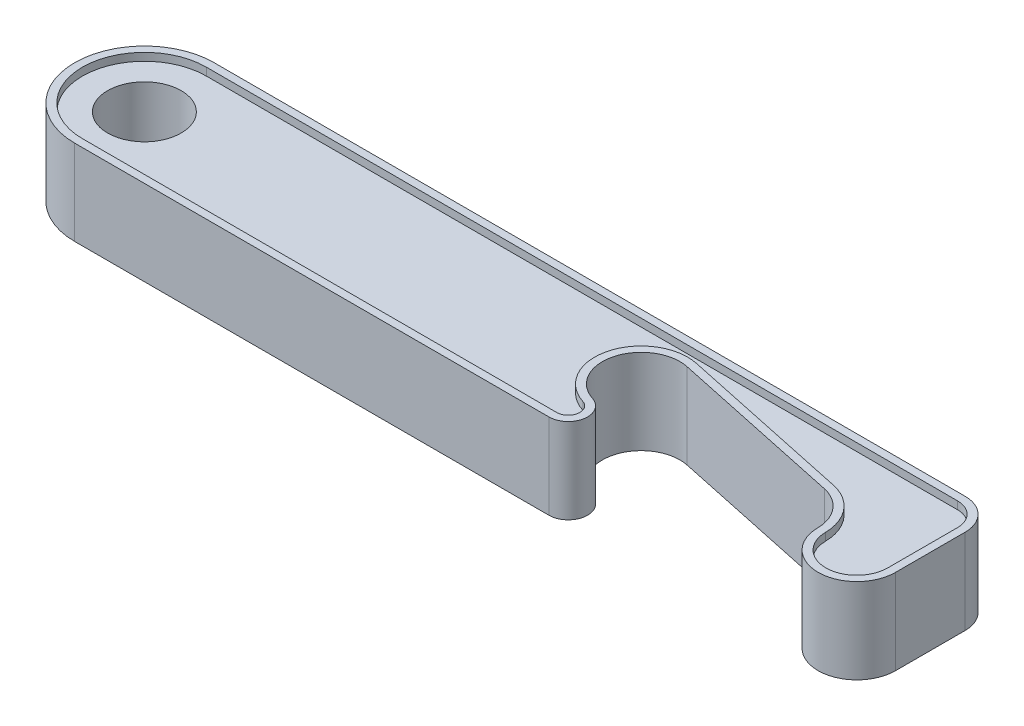
ISO-10303-21;
HEADER;
FILE_DESCRIPTION(('STEP AP214'),'2;1');
FILE_NAME('part.step','',(''),(''),'','','');
FILE_SCHEMA(('AUTOMOTIVE_DESIGN { 1 0 10303 214 1 1 1 1 }'));
ENDSEC;
DATA;
#1=APPLICATION_CONTEXT('core data for automotive mechanical design processes');
#2=APPLICATION_PROTOCOL_DEFINITION('international standard','automotive_design',2000,#1);
#3=PRODUCT_CONTEXT('',#1,'mechanical');
#4=PRODUCT('Part','Part','',(#3));
#5=PRODUCT_RELATED_PRODUCT_CATEGORY('part','',(#4));
#6=PRODUCT_DEFINITION_FORMATION('','',#4);
#7=PRODUCT_DEFINITION_CONTEXT('part definition',#1,'design');
#8=PRODUCT_DEFINITION('design','',#6,#7);
#9=PRODUCT_DEFINITION_SHAPE('','',#8);
#10=(LENGTH_UNIT() NAMED_UNIT(*) SI_UNIT(.MILLI.,.METRE.));
#11=(NAMED_UNIT(*) PLANE_ANGLE_UNIT() SI_UNIT($,.RADIAN.));
#12=(NAMED_UNIT(*) SI_UNIT($,.STERADIAN.) SOLID_ANGLE_UNIT());
#13=UNCERTAINTY_MEASURE_WITH_UNIT(LENGTH_MEASURE(1.E-05),#10,'distance_accuracy_value','');
#14=(GEOMETRIC_REPRESENTATION_CONTEXT(3) GLOBAL_UNCERTAINTY_ASSIGNED_CONTEXT((#13)) GLOBAL_UNIT_ASSIGNED_CONTEXT((#10,
#11,#12)) REPRESENTATION_CONTEXT('',''));
#15=CARTESIAN_POINT('',(0.,0.,0.));
#16=DIRECTION('',(0.,0.,1.));
#17=DIRECTION('',(1.,0.,0.));
#18=AXIS2_PLACEMENT_3D('',#15,#16,#17);
#19=CARTESIAN_POINT('',(0.,4.5,0.));
#20=DIRECTION('',(0.,-1.,0.));
#21=DIRECTION('',(0.,0.,-1.));
#22=AXIS2_PLACEMENT_3D('',#19,#20,#21);
#23=CYLINDRICAL_SURFACE('',#22,4.75);
#24=CARTESIAN_POINT('',(0.,4.5,0.));
#25=DIRECTION('',(0.,1.,0.));
#26=DIRECTION('',(0.,0.,1.));
#27=AXIS2_PLACEMENT_3D('',#24,#25,#26);
#28=CIRCLE('',#27,4.75);
#29=CARTESIAN_POINT('',(0.,4.5,4.75));
#30=VERTEX_POINT('',#29);
#31=EDGE_CURVE('E97',#30,#30,#28,.T.);
#32=ORIENTED_EDGE('',*,*,#31,.T.);
#33=EDGE_LOOP('',(#32));
#34=FACE_BOUND('',#33,.T.);
#35=CARTESIAN_POINT('',(0.,-4.5,0.));
#36=DIRECTION('',(0.,1.,0.));
#37=DIRECTION('',(0.,0.,1.));
#38=AXIS2_PLACEMENT_3D('',#35,#36,#37);
#39=CIRCLE('',#38,4.75);
#40=CARTESIAN_POINT('',(0.,-4.5,4.75));
#41=VERTEX_POINT('',#40);
#42=EDGE_CURVE('E159',#41,#41,#39,.T.);
#43=ORIENTED_EDGE('',*,*,#42,.F.);
#44=EDGE_LOOP('',(#43));
#45=FACE_BOUND('',#44,.T.);
#46=ADVANCED_FACE('F41',(#34,#45),#23,.F.);
#47=CARTESIAN_POINT('',(0.,4.5,0.));
#48=DIRECTION('',(0.,1.,0.));
#49=DIRECTION('',(0.,0.,1.));
#50=AXIS2_PLACEMENT_3D('',#47,#48,#49);
#51=PLANE('',#50);
#52=ORIENTED_EDGE('',*,*,#31,.F.);
#53=EDGE_LOOP('',(#52));
#54=FACE_BOUND('',#53,.T.);
#55=CARTESIAN_POINT('',(86.0008864599619,4.5,4.13314808832979));
#56=DIRECTION('',(0.,1.,0.));
#57=DIRECTION('',(0.,0.,1.));
#58=AXIS2_PLACEMENT_3D('',#55,#56,#57);
#59=CIRCLE('',#58,6.);
#60=CARTESIAN_POINT('',(92.0003545839848,4.5,4.05325923533293));
#61=VERTEX_POINT('',#60);
#62=CARTESIAN_POINT('',(87.2483566048684,4.5,-1.73573751607304));
#63=VERTEX_POINT('',#62);
#64=EDGE_CURVE('E133',#61,#63,#59,.T.);
#65=ORIENTED_EDGE('',*,*,#64,.F.);
#66=CARTESIAN_POINT('',(96.,4.5,4.));
#67=DIRECTION('',(0.,1.,0.));
#68=DIRECTION('',(0.,0.,1.));
#69=AXIS2_PLACEMENT_3D('',#66,#67,#68);
#70=CIRCLE('',#69,4.);
#71=CARTESIAN_POINT('',(100.,4.5,3.99999999999996));
#72=VERTEX_POINT('',#71);
#73=EDGE_CURVE('E140',#61,#72,#70,.T.);
#74=ORIENTED_EDGE('',*,*,#73,.T.);
#75=DIRECTION('',(0.,0.,-1.));
#76=VECTOR('',#75,1.);
#77=CARTESIAN_POINT('',(100.,4.5,0.));
#78=LINE('',#77,#76);
#79=CARTESIAN_POINT('',(100.,4.5,-4.99999999999997));
#80=VERTEX_POINT('',#79);
#81=EDGE_CURVE('E136',#72,#80,#78,.T.);
#82=ORIENTED_EDGE('',*,*,#81,.T.);
#83=CARTESIAN_POINT('',(97.,4.5,-5.));
#84=DIRECTION('',(0.,1.,0.));
#85=DIRECTION('',(0.,0.,1.));
#86=AXIS2_PLACEMENT_3D('',#83,#84,#85);
#87=CIRCLE('',#86,3.);
#88=CARTESIAN_POINT('',(97.,4.5,-8.));
#89=VERTEX_POINT('',#88);
#90=EDGE_CURVE('E141',#80,#89,#87,.T.);
#91=ORIENTED_EDGE('',*,*,#90,.T.);
#92=DIRECTION('',(1.,0.,0.));
#93=VECTOR('',#92,1.);
#94=CARTESIAN_POINT('',(0.,4.5,-8.));
#95=LINE('',#94,#93);
#96=CARTESIAN_POINT('',(0.,4.5,-8.));
#97=VERTEX_POINT('',#96);
#98=EDGE_CURVE('E148',#97,#89,#95,.T.);
#99=ORIENTED_EDGE('',*,*,#98,.F.);
#100=CARTESIAN_POINT('',(0.,4.5,0.));
#101=DIRECTION('',(0.,1.,0.));
#102=DIRECTION('',(0.,0.,1.));
#103=AXIS2_PLACEMENT_3D('',#100,#101,#102);
#104=CIRCLE('',#103,8.);
#105=CARTESIAN_POINT('',(0.,4.5,8.));
#106=VERTEX_POINT('',#105);
#107=EDGE_CURVE('E149',#97,#106,#104,.T.);
#108=ORIENTED_EDGE('',*,*,#107,.T.);
#109=DIRECTION('',(1.,0.,0.));
#110=VECTOR('',#109,1.);
#111=CARTESIAN_POINT('',(0.,4.5,8.));
#112=LINE('',#111,#110);
#113=CARTESIAN_POINT('',(61.234514126342,4.5,8.));
#114=VERTEX_POINT('',#113);
#115=EDGE_CURVE('E155',#106,#114,#112,.T.);
#116=ORIENTED_EDGE('',*,*,#115,.T.);
#117=CARTESIAN_POINT('',(61.234514126342,4.5,6.5));
#118=DIRECTION('',(0.,1.,0.));
#119=DIRECTION('',(0.,0.,1.));
#120=AXIS2_PLACEMENT_3D('',#117,#118,#119);
#121=CIRCLE('',#120,1.5);
#122=CARTESIAN_POINT('',(61.687788593066,4.5,5.07012509015086));
#123=VERTEX_POINT('',#122);
#124=EDGE_CURVE('E154',#114,#123,#121,.T.);
#125=ORIENTED_EDGE('',*,*,#124,.T.);
#126=CARTESIAN_POINT('',(63.5008864599619,4.5,-0.649374549245707));
#127=DIRECTION('',(0.,1.,0.));
#128=DIRECTION('',(0.,0.,1.));
#129=AXIS2_PLACEMENT_3D('',#126,#127,#128);
#130=CIRCLE('',#129,6.);
#131=CARTESIAN_POINT('',(64.7483566048684,4.5,-6.51826015364854));
#132=VERTEX_POINT('',#131);
#133=EDGE_CURVE('E49',#132,#123,#130,.T.);
#134=ORIENTED_EDGE('',*,*,#133,.F.);
#135=DIRECTION('',(0.978147600733806,0.,0.20791169081776));
#136=VECTOR('',#135,1.);
#137=CARTESIAN_POINT('',(4.12450239612868,4.5,-19.404258159443));
#138=LINE('',#137,#136);
#139=EDGE_CURVE('E11',#132,#63,#138,.T.);
#140=ORIENTED_EDGE('',*,*,#139,.T.);
#141=EDGE_LOOP('',(#65,#74,#82,#91,#99,#108,#116,#125,#134,#140));
#142=FACE_BOUND('',#141,.T.);
#143=ADVANCED_FACE('F232',(#54,#142),#51,.T.);
#144=CARTESIAN_POINT('',(0.,-4.5,0.));
#145=DIRECTION('',(0.,1.,0.));
#146=DIRECTION('',(0.,0.,1.));
#147=AXIS2_PLACEMENT_3D('',#144,#145,#146);
#148=PLANE('',#147);
#149=ORIENTED_EDGE('',*,*,#42,.T.);
#150=EDGE_LOOP('',(#149));
#151=FACE_BOUND('',#150,.T.);
#152=CARTESIAN_POINT('',(86.0008864599619,-4.5,4.13314808832979));
#153=DIRECTION('',(0.,1.,0.));
#154=DIRECTION('',(0.,0.,1.));
#155=AXIS2_PLACEMENT_3D('',#152,#153,#154);
#156=CIRCLE('',#155,6.);
#157=CARTESIAN_POINT('',(92.0003545839848,-4.5,4.05325923533293));
#158=VERTEX_POINT('',#157);
#159=CARTESIAN_POINT('',(87.2483566048684,-4.5,-1.73573751607304));
#160=VERTEX_POINT('',#159);
#161=EDGE_CURVE('E94',#158,#160,#156,.T.);
#162=ORIENTED_EDGE('',*,*,#161,.T.);
#163=DIRECTION('',(0.978147600733806,0.,0.20791169081776));
#164=VECTOR('',#163,1.);
#165=CARTESIAN_POINT('',(4.12450239612868,-4.5,-19.404258159443));
#166=LINE('',#165,#164);
#167=CARTESIAN_POINT('',(64.7483566048684,-4.5,-6.51826015364854));
#168=VERTEX_POINT('',#167);
#169=EDGE_CURVE('E42',#168,#160,#166,.T.);
#170=ORIENTED_EDGE('',*,*,#169,.F.);
#171=CARTESIAN_POINT('',(63.5008864599619,-4.5,-0.649374549245707));
#172=DIRECTION('',(0.,1.,0.));
#173=DIRECTION('',(0.,0.,1.));
#174=AXIS2_PLACEMENT_3D('',#171,#172,#173);
#175=CIRCLE('',#174,6.);
#176=CARTESIAN_POINT('',(61.687788593066,-4.5,5.07012509015086));
#177=VERTEX_POINT('',#176);
#178=EDGE_CURVE('E93',#168,#177,#175,.T.);
#179=ORIENTED_EDGE('',*,*,#178,.T.);
#180=CARTESIAN_POINT('',(61.234514126342,-4.5,6.5));
#181=DIRECTION('',(0.,1.,0.));
#182=DIRECTION('',(0.,0.,1.));
#183=AXIS2_PLACEMENT_3D('',#180,#181,#182);
#184=CIRCLE('',#183,1.5);
#185=CARTESIAN_POINT('',(61.234514126342,-4.5,8.));
#186=VERTEX_POINT('',#185);
#187=EDGE_CURVE('E109',#186,#177,#184,.T.);
#188=ORIENTED_EDGE('',*,*,#187,.F.);
#189=DIRECTION('',(1.,0.,0.));
#190=VECTOR('',#189,1.);
#191=CARTESIAN_POINT('',(0.,-4.5,8.));
#192=LINE('',#191,#190);
#193=CARTESIAN_POINT('',(0.,-4.5,8.));
#194=VERTEX_POINT('',#193);
#195=EDGE_CURVE('E179',#194,#186,#192,.T.);
#196=ORIENTED_EDGE('',*,*,#195,.F.);
#197=CARTESIAN_POINT('',(0.,-4.5,0.));
#198=DIRECTION('',(0.,1.,0.));
#199=DIRECTION('',(0.,0.,1.));
#200=AXIS2_PLACEMENT_3D('',#197,#198,#199);
#201=CIRCLE('',#200,8.);
#202=CARTESIAN_POINT('',(0.,-4.5,-8.));
#203=VERTEX_POINT('',#202);
#204=EDGE_CURVE('E177',#203,#194,#201,.T.);
#205=ORIENTED_EDGE('',*,*,#204,.F.);
#206=DIRECTION('',(1.,0.,0.));
#207=VECTOR('',#206,1.);
#208=CARTESIAN_POINT('',(0.,-4.5,-8.));
#209=LINE('',#208,#207);
#210=CARTESIAN_POINT('',(97.,-4.5,-8.));
#211=VERTEX_POINT('',#210);
#212=EDGE_CURVE('E173',#203,#211,#209,.T.);
#213=ORIENTED_EDGE('',*,*,#212,.T.);
#214=CARTESIAN_POINT('',(97.,-4.5,-5.));
#215=DIRECTION('',(0.,1.,0.));
#216=DIRECTION('',(0.,0.,1.));
#217=AXIS2_PLACEMENT_3D('',#214,#215,#216);
#218=CIRCLE('',#217,3.);
#219=CARTESIAN_POINT('',(100.,-4.5,-4.99999999999997));
#220=VERTEX_POINT('',#219);
#221=EDGE_CURVE('E171',#220,#211,#218,.T.);
#222=ORIENTED_EDGE('',*,*,#221,.F.);
#223=DIRECTION('',(0.,0.,-1.));
#224=VECTOR('',#223,1.);
#225=CARTESIAN_POINT('',(100.,-4.5,0.));
#226=LINE('',#225,#224);
#227=CARTESIAN_POINT('',(100.,-4.5,3.99999999999996));
#228=VERTEX_POINT('',#227);
#229=EDGE_CURVE('E169',#228,#220,#226,.T.);
#230=ORIENTED_EDGE('',*,*,#229,.F.);
#231=CARTESIAN_POINT('',(96.,-4.5,4.));
#232=DIRECTION('',(0.,1.,0.));
#233=DIRECTION('',(0.,0.,1.));
#234=AXIS2_PLACEMENT_3D('',#231,#232,#233);
#235=CIRCLE('',#234,4.);
#236=EDGE_CURVE('E164',#158,#228,#235,.T.);
#237=ORIENTED_EDGE('',*,*,#236,.F.);
#238=EDGE_LOOP('',(#162,#170,#179,#188,#196,#205,#213,#222,#230,#237));
#239=FACE_BOUND('',#238,.T.);
#240=ADVANCED_FACE('F89',(#151,#239),#148,.F.);
#241=CARTESIAN_POINT('',(96.,5.5,4.));
#242=DIRECTION('',(0.,-1.,0.));
#243=DIRECTION('',(0.,0.,-1.));
#244=AXIS2_PLACEMENT_3D('',#241,#242,#243);
#245=CYLINDRICAL_SURFACE('',#244,4.);
#246=ORIENTED_EDGE('',*,*,#236,.T.);
#247=DIRECTION('',(0.,-1.,0.));
#248=VECTOR('',#247,1.);
#249=CARTESIAN_POINT('',(100.,5.5,3.99999999999996));
#250=LINE('',#249,#248);
#251=CARTESIAN_POINT('',(100.,-5.5,3.99999999999996));
#252=VERTEX_POINT('',#251);
#253=EDGE_CURVE('E303',#228,#252,#250,.T.);
#254=ORIENTED_EDGE('',*,*,#253,.T.);
#255=CARTESIAN_POINT('',(96.,-5.5,4.));
#256=DIRECTION('',(0.,1.,0.));
#257=DIRECTION('',(0.,0.,1.));
#258=AXIS2_PLACEMENT_3D('',#255,#256,#257);
#259=CIRCLE('',#258,4.);
#260=CARTESIAN_POINT('',(92.0003545839848,-5.5,4.05325923533293));
#261=VERTEX_POINT('',#260);
#262=EDGE_CURVE('E304',#261,#252,#259,.T.);
#263=ORIENTED_EDGE('',*,*,#262,.F.);
#264=DIRECTION('',(0.,-1.,0.));
#265=VECTOR('',#264,1.);
#266=CARTESIAN_POINT('',(92.0003545839848,5.5,4.05325923533293));
#267=LINE('',#266,#265);
#268=EDGE_CURVE('E130',#158,#261,#267,.T.);
#269=ORIENTED_EDGE('',*,*,#268,.F.);
#270=EDGE_LOOP('',(#246,#254,#263,#269));
#271=FACE_BOUND('',#270,.T.);
#272=ADVANCED_FACE('F545',(#271),#245,.F.);
#273=CARTESIAN_POINT('',(86.0008864599619,5.5,4.13314808832979));
#274=DIRECTION('',(0.,-1.,0.));
#275=DIRECTION('',(0.,0.,-1.));
#276=AXIS2_PLACEMENT_3D('',#273,#274,#275);
#277=CYLINDRICAL_SURFACE('',#276,6.);
#278=DIRECTION('',(0.,-1.,0.));
#279=VECTOR('',#278,1.);
#280=CARTESIAN_POINT('',(87.2483566048684,5.5,-1.73573751607304));
#281=LINE('',#280,#279);
#282=CARTESIAN_POINT('',(87.2483566048684,-5.5,-1.73573751607304));
#283=VERTEX_POINT('',#282);
#284=EDGE_CURVE('E118',#160,#283,#281,.T.);
#285=ORIENTED_EDGE('',*,*,#284,.F.);
#286=ORIENTED_EDGE('',*,*,#161,.F.);
#287=ORIENTED_EDGE('',*,*,#268,.T.);
#288=CARTESIAN_POINT('',(86.0008864599619,-5.5,4.13314808832979));
#289=DIRECTION('',(0.,1.,0.));
#290=DIRECTION('',(0.,0.,1.));
#291=AXIS2_PLACEMENT_3D('',#288,#289,#290);
#292=CIRCLE('',#291,6.);
#293=EDGE_CURVE('E307',#261,#283,#292,.T.);
#294=ORIENTED_EDGE('',*,*,#293,.T.);
#295=EDGE_LOOP('',(#285,#286,#287,#294));
#296=FACE_BOUND('',#295,.T.);
#297=ADVANCED_FACE('F537',(#296),#277,.T.);
#298=CARTESIAN_POINT('',(4.12450239612868,5.5,-19.404258159443));
#299=DIRECTION('',(0.20791169081776,0.,-0.978147600733806));
#300=DIRECTION('',(-0.978147600733806,0.,-0.20791169081776));
#301=AXIS2_PLACEMENT_3D('',#298,#299,#300);
#302=PLANE('',#301);
#303=ORIENTED_EDGE('',*,*,#169,.T.);
#304=ORIENTED_EDGE('',*,*,#284,.T.);
#305=DIRECTION('',(0.978147600733806,0.,0.20791169081776));
#306=VECTOR('',#305,1.);
#307=CARTESIAN_POINT('',(4.12450239612868,-5.5,-19.404258159443));
#308=LINE('',#307,#306);
#309=CARTESIAN_POINT('',(64.7483566048684,-5.5,-6.51826015364854));
#310=VERTEX_POINT('',#309);
#311=EDGE_CURVE('E111',#310,#283,#308,.T.);
#312=ORIENTED_EDGE('',*,*,#311,.F.);
#313=DIRECTION('',(0.,-1.,0.));
#314=VECTOR('',#313,1.);
#315=CARTESIAN_POINT('',(64.7483566048684,5.5,-6.51826015364854));
#316=LINE('',#315,#314);
#317=EDGE_CURVE('E106',#168,#310,#316,.T.);
#318=ORIENTED_EDGE('',*,*,#317,.F.);
#319=EDGE_LOOP('',(#303,#304,#312,#318));
#320=FACE_BOUND('',#319,.T.);
#321=ADVANCED_FACE('F115',(#320),#302,.T.);
#322=CARTESIAN_POINT('',(63.5008864599619,5.5,-0.649374549245707));
#323=DIRECTION('',(0.,-1.,0.));
#324=DIRECTION('',(0.,0.,-1.));
#325=AXIS2_PLACEMENT_3D('',#322,#323,#324);
#326=CYLINDRICAL_SURFACE('',#325,6.);
#327=DIRECTION('',(0.,-1.,0.));
#328=VECTOR('',#327,1.);
#329=CARTESIAN_POINT('',(61.687788593066,5.5,5.07012509015086));
#330=LINE('',#329,#328);
#331=CARTESIAN_POINT('',(61.687788593066,-5.5,5.07012509015086));
#332=VERTEX_POINT('',#331);
#333=EDGE_CURVE('E108',#177,#332,#330,.T.);
#334=ORIENTED_EDGE('',*,*,#333,.F.);
#335=ORIENTED_EDGE('',*,*,#178,.F.);
#336=ORIENTED_EDGE('',*,*,#317,.T.);
#337=CARTESIAN_POINT('',(63.5008864599619,-5.5,-0.649374549245707));
#338=DIRECTION('',(0.,1.,0.));
#339=DIRECTION('',(0.,0.,1.));
#340=AXIS2_PLACEMENT_3D('',#337,#338,#339);
#341=CIRCLE('',#340,6.);
#342=EDGE_CURVE('E313',#310,#332,#341,.T.);
#343=ORIENTED_EDGE('',*,*,#342,.T.);
#344=EDGE_LOOP('',(#334,#335,#336,#343));
#345=FACE_BOUND('',#344,.T.);
#346=ADVANCED_FACE('F103',(#345),#326,.T.);
#347=CARTESIAN_POINT('',(61.234514126342,5.5,6.5));
#348=DIRECTION('',(0.,-1.,0.));
#349=DIRECTION('',(0.,0.,-1.));
#350=AXIS2_PLACEMENT_3D('',#347,#348,#349);
#351=CYLINDRICAL_SURFACE('',#350,1.5);
#352=ORIENTED_EDGE('',*,*,#187,.T.);
#353=ORIENTED_EDGE('',*,*,#333,.T.);
#354=CARTESIAN_POINT('',(61.234514126342,-5.5,6.5));
#355=DIRECTION('',(0.,1.,0.));
#356=DIRECTION('',(0.,0.,1.));
#357=AXIS2_PLACEMENT_3D('',#354,#355,#356);
#358=CIRCLE('',#357,1.5);
#359=CARTESIAN_POINT('',(61.234514126342,-5.5,8.));
#360=VERTEX_POINT('',#359);
#361=EDGE_CURVE('E311',#360,#332,#358,.T.);
#362=ORIENTED_EDGE('',*,*,#361,.F.);
#363=DIRECTION('',(0.,-1.,0.));
#364=VECTOR('',#363,1.);
#365=CARTESIAN_POINT('',(61.234514126342,5.5,8.));
#366=LINE('',#365,#364);
#367=EDGE_CURVE('E187',#186,#360,#366,.T.);
#368=ORIENTED_EDGE('',*,*,#367,.F.);
#369=EDGE_LOOP('',(#352,#353,#362,#368));
#370=FACE_BOUND('',#369,.T.);
#371=ADVANCED_FACE('F184',(#370),#351,.F.);
#372=CARTESIAN_POINT('',(0.,5.5,8.));
#373=DIRECTION('',(0.,0.,-1.));
#374=DIRECTION('',(-1.,0.,0.));
#375=AXIS2_PLACEMENT_3D('',#372,#373,#374);
#376=PLANE('',#375);
#377=ORIENTED_EDGE('',*,*,#195,.T.);
#378=ORIENTED_EDGE('',*,*,#367,.T.);
#379=DIRECTION('',(1.,0.,0.));
#380=VECTOR('',#379,1.);
#381=CARTESIAN_POINT('',(0.,-5.5,8.));
#382=LINE('',#381,#380);
#383=CARTESIAN_POINT('',(0.,-5.5,8.));
#384=VERTEX_POINT('',#383);
#385=EDGE_CURVE('E196',#384,#360,#382,.T.);
#386=ORIENTED_EDGE('',*,*,#385,.F.);
#387=DIRECTION('',(0.,-1.,0.));
#388=VECTOR('',#387,1.);
#389=CARTESIAN_POINT('',(0.,5.5,8.));
#390=LINE('',#389,#388);
#391=EDGE_CURVE('E191',#194,#384,#390,.T.);
#392=ORIENTED_EDGE('',*,*,#391,.F.);
#393=EDGE_LOOP('',(#377,#378,#386,#392));
#394=FACE_BOUND('',#393,.T.);
#395=ADVANCED_FACE('F192',(#394),#376,.T.);
#396=CARTESIAN_POINT('',(0.,5.5,0.));
#397=DIRECTION('',(0.,-1.,0.));
#398=DIRECTION('',(0.,0.,-1.));
#399=AXIS2_PLACEMENT_3D('',#396,#397,#398);
#400=CYLINDRICAL_SURFACE('',#399,8.);
#401=ORIENTED_EDGE('',*,*,#204,.T.);
#402=ORIENTED_EDGE('',*,*,#391,.T.);
#403=CARTESIAN_POINT('',(0.,-5.5,0.));
#404=DIRECTION('',(0.,1.,0.));
#405=DIRECTION('',(0.,0.,1.));
#406=AXIS2_PLACEMENT_3D('',#403,#404,#405);
#407=CIRCLE('',#406,8.);
#408=CARTESIAN_POINT('',(0.,-5.5,-8.));
#409=VERTEX_POINT('',#408);
#410=EDGE_CURVE('E320',#409,#384,#407,.T.);
#411=ORIENTED_EDGE('',*,*,#410,.F.);
#412=DIRECTION('',(0.,-1.,0.));
#413=VECTOR('',#412,1.);
#414=CARTESIAN_POINT('',(0.,5.5,-8.));
#415=LINE('',#414,#413);
#416=EDGE_CURVE('E210',#203,#409,#415,.T.);
#417=ORIENTED_EDGE('',*,*,#416,.F.);
#418=EDGE_LOOP('',(#401,#402,#411,#417));
#419=FACE_BOUND('',#418,.T.);
#420=ADVANCED_FACE('F541',(#419),#400,.F.);
#421=CARTESIAN_POINT('',(0.,5.5,-8.));
#422=DIRECTION('',(0.,0.,-1.));
#423=DIRECTION('',(-1.,0.,0.));
#424=AXIS2_PLACEMENT_3D('',#421,#422,#423);
#425=PLANE('',#424);
#426=DIRECTION('',(0.,-1.,0.));
#427=VECTOR('',#426,1.);
#428=CARTESIAN_POINT('',(97.,5.5,-8.));
#429=LINE('',#428,#427);
#430=CARTESIAN_POINT('',(97.,-5.5,-8.));
#431=VERTEX_POINT('',#430);
#432=EDGE_CURVE('E391',#211,#431,#429,.T.);
#433=ORIENTED_EDGE('',*,*,#432,.F.);
#434=ORIENTED_EDGE('',*,*,#212,.F.);
#435=ORIENTED_EDGE('',*,*,#416,.T.);
#436=DIRECTION('',(1.,0.,0.));
#437=VECTOR('',#436,1.);
#438=CARTESIAN_POINT('',(0.,-5.5,-8.));
#439=LINE('',#438,#437);
#440=EDGE_CURVE('E317',#409,#431,#439,.T.);
#441=ORIENTED_EDGE('',*,*,#440,.T.);
#442=EDGE_LOOP('',(#433,#434,#435,#441));
#443=FACE_BOUND('',#442,.T.);
#444=ADVANCED_FACE('F407',(#443),#425,.F.);
#445=CARTESIAN_POINT('',(97.,5.5,-5.));
#446=DIRECTION('',(0.,-1.,0.));
#447=DIRECTION('',(0.,0.,-1.));
#448=AXIS2_PLACEMENT_3D('',#445,#446,#447);
#449=CYLINDRICAL_SURFACE('',#448,3.);
#450=ORIENTED_EDGE('',*,*,#221,.T.);
#451=ORIENTED_EDGE('',*,*,#432,.T.);
#452=CARTESIAN_POINT('',(97.,-5.5,-5.));
#453=DIRECTION('',(0.,1.,0.));
#454=DIRECTION('',(0.,0.,1.));
#455=AXIS2_PLACEMENT_3D('',#452,#453,#454);
#456=CIRCLE('',#455,3.);
#457=CARTESIAN_POINT('',(100.,-5.5,-4.99999999999997));
#458=VERTEX_POINT('',#457);
#459=EDGE_CURVE('E325',#458,#431,#456,.T.);
#460=ORIENTED_EDGE('',*,*,#459,.F.);
#461=DIRECTION('',(0.,-1.,0.));
#462=VECTOR('',#461,1.);
#463=CARTESIAN_POINT('',(100.,5.5,-4.99999999999997));
#464=LINE('',#463,#462);
#465=EDGE_CURVE('E388',#220,#458,#464,.T.);
#466=ORIENTED_EDGE('',*,*,#465,.F.);
#467=EDGE_LOOP('',(#450,#451,#460,#466));
#468=FACE_BOUND('',#467,.T.);
#469=ADVANCED_FACE('F399',(#468),#449,.F.);
#470=CARTESIAN_POINT('',(100.,5.5,0.));
#471=DIRECTION('',(-1.,0.,0.));
#472=DIRECTION('',(0.,0.,1.));
#473=AXIS2_PLACEMENT_3D('',#470,#471,#472);
#474=PLANE('',#473);
#475=ORIENTED_EDGE('',*,*,#229,.T.);
#476=ORIENTED_EDGE('',*,*,#465,.T.);
#477=DIRECTION('',(0.,0.,-1.));
#478=VECTOR('',#477,1.);
#479=CARTESIAN_POINT('',(100.,-5.5,0.));
#480=LINE('',#479,#478);
#481=EDGE_CURVE('E324',#252,#458,#480,.T.);
#482=ORIENTED_EDGE('',*,*,#481,.F.);
#483=ORIENTED_EDGE('',*,*,#253,.F.);
#484=EDGE_LOOP('',(#475,#476,#482,#483));
#485=FACE_BOUND('',#484,.T.);
#486=ADVANCED_FACE('F423',(#485),#474,.T.);
#487=CARTESIAN_POINT('',(86.0008864599619,5.5,4.13314808832979));
#488=DIRECTION('',(0.,-1.,0.));
#489=DIRECTION('',(0.,0.,-1.));
#490=AXIS2_PLACEMENT_3D('',#487,#488,#489);
#491=CYLINDRICAL_SURFACE('',#490,5.);
#492=CARTESIAN_POINT('',(86.0008864599619,-5.5,4.13314808832979));
#493=DIRECTION('',(0.,1.,0.));
#494=DIRECTION('',(0.,0.,1.));
#495=AXIS2_PLACEMENT_3D('',#492,#493,#494);
#496=CIRCLE('',#495,5.);
#497=CARTESIAN_POINT('',(91.0004432299809,-5.5,4.06657404416574));
#498=VERTEX_POINT('',#497);
#499=CARTESIAN_POINT('',(87.0404449140507,-5.5,-0.757589915339231));
#500=VERTEX_POINT('',#499);
#501=EDGE_CURVE('E327',#498,#500,#496,.T.);
#502=ORIENTED_EDGE('',*,*,#501,.F.);
#503=DIRECTION('',(0.,-1.,0.));
#504=VECTOR('',#503,1.);
#505=CARTESIAN_POINT('',(91.0004432299809,5.5,4.06657404416574));
#506=LINE('',#505,#504);
#507=CARTESIAN_POINT('',(91.0004432299809,5.5,4.06657404416574));
#508=VERTEX_POINT('',#507);
#509=EDGE_CURVE('E162',#508,#498,#506,.T.);
#510=ORIENTED_EDGE('',*,*,#509,.F.);
#511=CARTESIAN_POINT('',(86.0008864599619,5.5,4.13314808832979));
#512=DIRECTION('',(0.,1.,0.));
#513=DIRECTION('',(0.,0.,1.));
#514=AXIS2_PLACEMENT_3D('',#511,#512,#513);
#515=CIRCLE('',#514,5.);
#516=CARTESIAN_POINT('',(87.0404449140507,5.5,-0.757589915339231));
#517=VERTEX_POINT('',#516);
#518=EDGE_CURVE('E272',#508,#517,#515,.T.);
#519=ORIENTED_EDGE('',*,*,#518,.T.);
#520=DIRECTION('',(0.,-1.,0.));
#521=VECTOR('',#520,1.);
#522=CARTESIAN_POINT('',(87.0404449140507,5.5,-0.757589915339231));
#523=LINE('',#522,#521);
#524=EDGE_CURVE('E131',#517,#500,#523,.T.);
#525=ORIENTED_EDGE('',*,*,#524,.T.);
#526=EDGE_LOOP('',(#502,#510,#519,#525));
#527=FACE_BOUND('',#526,.T.);
#528=ADVANCED_FACE('F649',(#527),#491,.F.);
#529=CARTESIAN_POINT('',(96.,5.5,4.));
#530=DIRECTION('',(0.,-1.,0.));
#531=DIRECTION('',(0.,0.,-1.));
#532=AXIS2_PLACEMENT_3D('',#529,#530,#531);
#533=CYLINDRICAL_SURFACE('',#532,5.);
#534=CARTESIAN_POINT('',(96.,-5.5,4.));
#535=DIRECTION('',(0.,1.,0.));
#536=DIRECTION('',(0.,0.,1.));
#537=AXIS2_PLACEMENT_3D('',#534,#535,#536);
#538=CIRCLE('',#537,5.);
#539=CARTESIAN_POINT('',(101.,-5.5,3.99999999999996));
#540=VERTEX_POINT('',#539);
#541=EDGE_CURVE('E332',#498,#540,#538,.T.);
#542=ORIENTED_EDGE('',*,*,#541,.T.);
#543=DIRECTION('',(0.,-1.,0.));
#544=VECTOR('',#543,1.);
#545=CARTESIAN_POINT('',(101.,5.5,3.99999999999996));
#546=LINE('',#545,#544);
#547=CARTESIAN_POINT('',(101.,5.5,3.99999999999996));
#548=VERTEX_POINT('',#547);
#549=EDGE_CURVE('E385',#548,#540,#546,.T.);
#550=ORIENTED_EDGE('',*,*,#549,.F.);
#551=CARTESIAN_POINT('',(96.,5.5,4.));
#552=DIRECTION('',(0.,1.,0.));
#553=DIRECTION('',(0.,0.,1.));
#554=AXIS2_PLACEMENT_3D('',#551,#552,#553);
#555=CIRCLE('',#554,5.);
#556=EDGE_CURVE('E277',#508,#548,#555,.T.);
#557=ORIENTED_EDGE('',*,*,#556,.F.);
#558=ORIENTED_EDGE('',*,*,#509,.T.);
#559=EDGE_LOOP('',(#542,#550,#557,#558));
#560=FACE_BOUND('',#559,.T.);
#561=ADVANCED_FACE('F659',(#560),#533,.T.);
#562=CARTESIAN_POINT('',(101.,5.5,0.));
#563=DIRECTION('',(-1.,0.,0.));
#564=DIRECTION('',(0.,0.,1.));
#565=AXIS2_PLACEMENT_3D('',#562,#563,#564);
#566=PLANE('',#565);
#567=DIRECTION('',(0.,0.,-1.));
#568=VECTOR('',#567,1.);
#569=CARTESIAN_POINT('',(101.,-5.5,0.));
#570=LINE('',#569,#568);
#571=CARTESIAN_POINT('',(101.,-5.5,-4.99999999999997));
#572=VERTEX_POINT('',#571);
#573=EDGE_CURVE('E331',#540,#572,#570,.T.);
#574=ORIENTED_EDGE('',*,*,#573,.T.);
#575=DIRECTION('',(0.,-1.,0.));
#576=VECTOR('',#575,1.);
#577=CARTESIAN_POINT('',(101.,5.5,-4.99999999999997));
#578=LINE('',#577,#576);
#579=CARTESIAN_POINT('',(101.,5.5,-4.99999999999997));
#580=VERTEX_POINT('',#579);
#581=EDGE_CURVE('E377',#580,#572,#578,.T.);
#582=ORIENTED_EDGE('',*,*,#581,.F.);
#583=DIRECTION('',(0.,0.,-1.));
#584=VECTOR('',#583,1.);
#585=CARTESIAN_POINT('',(101.,5.5,0.));
#586=LINE('',#585,#584);
#587=EDGE_CURVE('E276',#548,#580,#586,.T.);
#588=ORIENTED_EDGE('',*,*,#587,.F.);
#589=ORIENTED_EDGE('',*,*,#549,.T.);
#590=EDGE_LOOP('',(#574,#582,#588,#589));
#591=FACE_BOUND('',#590,.T.);
#592=ADVANCED_FACE('F669',(#591),#566,.F.);
#593=CARTESIAN_POINT('',(97.,5.5,-5.));
#594=DIRECTION('',(0.,-1.,0.));
#595=DIRECTION('',(0.,0.,-1.));
#596=AXIS2_PLACEMENT_3D('',#593,#594,#595);
#597=CYLINDRICAL_SURFACE('',#596,4.);
#598=CARTESIAN_POINT('',(97.,-5.5,-5.));
#599=DIRECTION('',(0.,1.,0.));
#600=DIRECTION('',(0.,0.,1.));
#601=AXIS2_PLACEMENT_3D('',#598,#599,#600);
#602=CIRCLE('',#601,4.);
#603=CARTESIAN_POINT('',(97.,-5.5,-9.));
#604=VERTEX_POINT('',#603);
#605=EDGE_CURVE('E340',#572,#604,#602,.T.);
#606=ORIENTED_EDGE('',*,*,#605,.T.);
#607=DIRECTION('',(0.,-1.,0.));
#608=VECTOR('',#607,1.);
#609=CARTESIAN_POINT('',(97.,5.5,-9.));
#610=LINE('',#609,#608);
#611=CARTESIAN_POINT('',(97.,5.5,-9.));
#612=VERTEX_POINT('',#611);
#613=EDGE_CURVE('E376',#612,#604,#610,.T.);
#614=ORIENTED_EDGE('',*,*,#613,.F.);
#615=CARTESIAN_POINT('',(97.,5.5,-5.));
#616=DIRECTION('',(0.,1.,0.));
#617=DIRECTION('',(0.,0.,1.));
#618=AXIS2_PLACEMENT_3D('',#615,#616,#617);
#619=CIRCLE('',#618,4.);
#620=EDGE_CURVE('E285',#580,#612,#619,.T.);
#621=ORIENTED_EDGE('',*,*,#620,.F.);
#622=ORIENTED_EDGE('',*,*,#581,.T.);
#623=EDGE_LOOP('',(#606,#614,#621,#622));
#624=FACE_BOUND('',#623,.T.);
#625=ADVANCED_FACE('F682',(#624),#597,.T.);
#626=CARTESIAN_POINT('',(0.,5.5,-9.));
#627=DIRECTION('',(0.,0.,-1.));
#628=DIRECTION('',(-1.,0.,0.));
#629=AXIS2_PLACEMENT_3D('',#626,#627,#628);
#630=PLANE('',#629);
#631=DIRECTION('',(1.,0.,0.));
#632=VECTOR('',#631,1.);
#633=CARTESIAN_POINT('',(0.,-5.5,-9.));
#634=LINE('',#633,#632);
#635=CARTESIAN_POINT('',(0.,-5.5,-9.));
#636=VERTEX_POINT('',#635);
#637=EDGE_CURVE('E339',#636,#604,#634,.T.);
#638=ORIENTED_EDGE('',*,*,#637,.F.);
#639=DIRECTION('',(0.,-1.,0.));
#640=VECTOR('',#639,1.);
#641=CARTESIAN_POINT('',(0.,5.5,-9.));
#642=LINE('',#641,#640);
#643=CARTESIAN_POINT('',(0.,5.5,-9.));
#644=VERTEX_POINT('',#643);
#645=EDGE_CURVE('E373',#644,#636,#642,.T.);
#646=ORIENTED_EDGE('',*,*,#645,.F.);
#647=DIRECTION('',(1.,0.,0.));
#648=VECTOR('',#647,1.);
#649=CARTESIAN_POINT('',(0.,5.5,-9.));
#650=LINE('',#649,#648);
#651=EDGE_CURVE('E284',#644,#612,#650,.T.);
#652=ORIENTED_EDGE('',*,*,#651,.T.);
#653=ORIENTED_EDGE('',*,*,#613,.T.);
#654=EDGE_LOOP('',(#638,#646,#652,#653));
#655=FACE_BOUND('',#654,.T.);
#656=ADVANCED_FACE('F691',(#655),#630,.T.);
#657=CARTESIAN_POINT('',(0.,5.5,0.));
#658=DIRECTION('',(0.,-1.,0.));
#659=DIRECTION('',(0.,0.,-1.));
#660=AXIS2_PLACEMENT_3D('',#657,#658,#659);
#661=CYLINDRICAL_SURFACE('',#660,9.);
#662=CARTESIAN_POINT('',(0.,-5.5,0.));
#663=DIRECTION('',(0.,1.,0.));
#664=DIRECTION('',(0.,0.,1.));
#665=AXIS2_PLACEMENT_3D('',#662,#663,#664);
#666=CIRCLE('',#665,9.);
#667=CARTESIAN_POINT('',(0.,-5.5,9.));
#668=VERTEX_POINT('',#667);
#669=EDGE_CURVE('E343',#636,#668,#666,.T.);
#670=ORIENTED_EDGE('',*,*,#669,.T.);
#671=DIRECTION('',(0.,-1.,0.));
#672=VECTOR('',#671,1.);
#673=CARTESIAN_POINT('',(0.,5.5,9.));
#674=LINE('',#673,#672);
#675=CARTESIAN_POINT('',(0.,5.5,9.));
#676=VERTEX_POINT('',#675);
#677=EDGE_CURVE('E367',#676,#668,#674,.T.);
#678=ORIENTED_EDGE('',*,*,#677,.F.);
#679=CARTESIAN_POINT('',(0.,5.5,0.));
#680=DIRECTION('',(0.,1.,0.));
#681=DIRECTION('',(0.,0.,1.));
#682=AXIS2_PLACEMENT_3D('',#679,#680,#681);
#683=CIRCLE('',#682,9.);
#684=EDGE_CURVE('E288',#644,#676,#683,.T.);
#685=ORIENTED_EDGE('',*,*,#684,.F.);
#686=ORIENTED_EDGE('',*,*,#645,.T.);
#687=EDGE_LOOP('',(#670,#678,#685,#686));
#688=FACE_BOUND('',#687,.T.);
#689=ADVANCED_FACE('F703',(#688),#661,.T.);
#690=CARTESIAN_POINT('',(0.,5.5,9.));
#691=DIRECTION('',(0.,0.,-1.));
#692=DIRECTION('',(-1.,0.,0.));
#693=AXIS2_PLACEMENT_3D('',#690,#691,#692);
#694=PLANE('',#693);
#695=DIRECTION('',(1.,0.,0.));
#696=VECTOR('',#695,1.);
#697=CARTESIAN_POINT('',(0.,-5.5,9.));
#698=LINE('',#697,#696);
#699=CARTESIAN_POINT('',(61.234514126342,-5.5,9.));
#700=VERTEX_POINT('',#699);
#701=EDGE_CURVE('E347',#668,#700,#698,.T.);
#702=ORIENTED_EDGE('',*,*,#701,.T.);
#703=DIRECTION('',(0.,-1.,0.));
#704=VECTOR('',#703,1.);
#705=CARTESIAN_POINT('',(61.234514126342,5.5,9.));
#706=LINE('',#705,#704);
#707=CARTESIAN_POINT('',(61.234514126342,5.5,9.));
#708=VERTEX_POINT('',#707);
#709=EDGE_CURVE('E370',#708,#700,#706,.T.);
#710=ORIENTED_EDGE('',*,*,#709,.F.);
#711=DIRECTION('',(1.,0.,0.));
#712=VECTOR('',#711,1.);
#713=CARTESIAN_POINT('',(0.,5.5,9.));
#714=LINE('',#713,#712);
#715=EDGE_CURVE('E292',#676,#708,#714,.T.);
#716=ORIENTED_EDGE('',*,*,#715,.F.);
#717=ORIENTED_EDGE('',*,*,#677,.T.);
#718=EDGE_LOOP('',(#702,#710,#716,#717));
#719=FACE_BOUND('',#718,.T.);
#720=ADVANCED_FACE('F712',(#719),#694,.F.);
#721=CARTESIAN_POINT('',(61.234514126342,5.5,6.5));
#722=DIRECTION('',(0.,-1.,0.));
#723=DIRECTION('',(0.,0.,-1.));
#724=AXIS2_PLACEMENT_3D('',#721,#722,#723);
#725=CYLINDRICAL_SURFACE('',#724,2.5);
#726=CARTESIAN_POINT('',(61.234514126342,-5.5,6.5));
#727=DIRECTION('',(0.,1.,0.));
#728=DIRECTION('',(0.,0.,1.));
#729=AXIS2_PLACEMENT_3D('',#726,#727,#728);
#730=CIRCLE('',#729,2.5);
#731=CARTESIAN_POINT('',(61.9899715708819,-5.5,4.11687515025143));
#732=VERTEX_POINT('',#731);
#733=EDGE_CURVE('E349',#700,#732,#730,.T.);
#734=ORIENTED_EDGE('',*,*,#733,.T.);
#735=DIRECTION('',(0.,-1.,0.));
#736=VECTOR('',#735,1.);
#737=CARTESIAN_POINT('',(61.9899715708819,5.5,4.11687515025143));
#738=LINE('',#737,#736);
#739=CARTESIAN_POINT('',(61.9899715708819,5.5,4.11687515025143));
#740=VERTEX_POINT('',#739);
#741=EDGE_CURVE('E365',#740,#732,#738,.T.);
#742=ORIENTED_EDGE('',*,*,#741,.F.);
#743=CARTESIAN_POINT('',(61.234514126342,5.5,6.5));
#744=DIRECTION('',(0.,1.,0.));
#745=DIRECTION('',(0.,0.,1.));
#746=AXIS2_PLACEMENT_3D('',#743,#744,#745);
#747=CIRCLE('',#746,2.5);
#748=EDGE_CURVE('E294',#708,#740,#747,.T.);
#749=ORIENTED_EDGE('',*,*,#748,.F.);
#750=ORIENTED_EDGE('',*,*,#709,.T.);
#751=EDGE_LOOP('',(#734,#742,#749,#750));
#752=FACE_BOUND('',#751,.T.);
#753=ADVANCED_FACE('F722',(#752),#725,.T.);
#754=CARTESIAN_POINT('',(63.5008864599619,5.5,-0.649374549245707));
#755=DIRECTION('',(0.,-1.,0.));
#756=DIRECTION('',(0.,0.,-1.));
#757=AXIS2_PLACEMENT_3D('',#754,#755,#756);
#758=CYLINDRICAL_SURFACE('',#757,5.);
#759=CARTESIAN_POINT('',(63.5008864599619,-5.5,-0.649374549245707));
#760=DIRECTION('',(0.,1.,0.));
#761=DIRECTION('',(0.,0.,1.));
#762=AXIS2_PLACEMENT_3D('',#759,#760,#761);
#763=CIRCLE('',#762,5.);
#764=CARTESIAN_POINT('',(64.5404449140507,-5.5,-5.54011255291474));
#765=VERTEX_POINT('',#764);
#766=EDGE_CURVE('E355',#765,#732,#763,.T.);
#767=ORIENTED_EDGE('',*,*,#766,.F.);
#768=DIRECTION('',(0.,-1.,0.));
#769=VECTOR('',#768,1.);
#770=CARTESIAN_POINT('',(64.5404449140507,5.5,-5.54011255291474));
#771=LINE('',#770,#769);
#772=CARTESIAN_POINT('',(64.5404449140507,5.5,-5.54011255291474));
#773=VERTEX_POINT('',#772);
#774=EDGE_CURVE('E363',#773,#765,#771,.T.);
#775=ORIENTED_EDGE('',*,*,#774,.F.);
#776=CARTESIAN_POINT('',(63.5008864599619,5.5,-0.649374549245707));
#777=DIRECTION('',(0.,1.,0.));
#778=DIRECTION('',(0.,0.,1.));
#779=AXIS2_PLACEMENT_3D('',#776,#777,#778);
#780=CIRCLE('',#779,5.);
#781=EDGE_CURVE('E300',#773,#740,#780,.T.);
#782=ORIENTED_EDGE('',*,*,#781,.T.);
#783=ORIENTED_EDGE('',*,*,#741,.T.);
#784=EDGE_LOOP('',(#767,#775,#782,#783));
#785=FACE_BOUND('',#784,.T.);
#786=ADVANCED_FACE('F554',(#785),#758,.F.);
#787=CARTESIAN_POINT('',(100.,5.5,3.99999999999996));
#788=VERTEX_POINT('',#787);
#789=EDGE_CURVE('E390',#788,#72,#250,.T.);
#790=ORIENTED_EDGE('',*,*,#789,.T.);
#791=ORIENTED_EDGE('',*,*,#73,.F.);
#792=CARTESIAN_POINT('',(92.0003545839848,5.5,4.05325923533293));
#793=VERTEX_POINT('',#792);
#794=EDGE_CURVE('E126',#793,#61,#267,.T.);
#795=ORIENTED_EDGE('',*,*,#794,.F.);
#796=CARTESIAN_POINT('',(96.,5.5,4.));
#797=DIRECTION('',(0.,1.,0.));
#798=DIRECTION('',(0.,0.,1.));
#799=AXIS2_PLACEMENT_3D('',#796,#797,#798);
#800=CIRCLE('',#799,4.);
#801=EDGE_CURVE('E358',#793,#788,#800,.T.);
#802=ORIENTED_EDGE('',*,*,#801,.T.);
#803=EDGE_LOOP('',(#790,#791,#795,#802));
#804=FACE_BOUND('',#803,.T.);
#805=ADVANCED_FACE('F467',(#804),#245,.F.);
#806=ORIENTED_EDGE('',*,*,#64,.T.);
#807=CARTESIAN_POINT('',(87.2483566048684,5.5,-1.73573751607304));
#808=VERTEX_POINT('',#807);
#809=EDGE_CURVE('E124',#808,#63,#281,.T.);
#810=ORIENTED_EDGE('',*,*,#809,.F.);
#811=CARTESIAN_POINT('',(86.0008864599619,5.5,4.13314808832979));
#812=DIRECTION('',(0.,1.,0.));
#813=DIRECTION('',(0.,0.,1.));
#814=AXIS2_PLACEMENT_3D('',#811,#812,#813);
#815=CIRCLE('',#814,6.);
#816=EDGE_CURVE('E472',#793,#808,#815,.T.);
#817=ORIENTED_EDGE('',*,*,#816,.F.);
#818=ORIENTED_EDGE('',*,*,#794,.T.);
#819=EDGE_LOOP('',(#806,#810,#817,#818));
#820=FACE_BOUND('',#819,.T.);
#821=ADVANCED_FACE('F466',(#820),#277,.T.);
#822=ORIENTED_EDGE('',*,*,#809,.T.);
#823=ORIENTED_EDGE('',*,*,#139,.F.);
#824=CARTESIAN_POINT('',(64.7483566048684,5.5,-6.51826015364854));
#825=VERTEX_POINT('',#824);
#826=EDGE_CURVE('E113',#825,#132,#316,.T.);
#827=ORIENTED_EDGE('',*,*,#826,.F.);
#828=DIRECTION('',(0.978147600733806,0.,0.20791169081776));
#829=VECTOR('',#828,1.);
#830=CARTESIAN_POINT('',(4.12450239612868,5.5,-19.404258159443));
#831=LINE('',#830,#829);
#832=EDGE_CURVE('E488',#825,#808,#831,.T.);
#833=ORIENTED_EDGE('',*,*,#832,.T.);
#834=EDGE_LOOP('',(#822,#823,#827,#833));
#835=FACE_BOUND('',#834,.T.);
#836=ADVANCED_FACE('F474',(#835),#302,.T.);
#837=ORIENTED_EDGE('',*,*,#133,.T.);
#838=CARTESIAN_POINT('',(61.687788593066,5.5,5.07012509015086));
#839=VERTEX_POINT('',#838);
#840=EDGE_CURVE('E116',#839,#123,#330,.T.);
#841=ORIENTED_EDGE('',*,*,#840,.F.);
#842=CARTESIAN_POINT('',(63.5008864599619,5.5,-0.649374549245707));
#843=DIRECTION('',(0.,1.,0.));
#844=DIRECTION('',(0.,0.,1.));
#845=AXIS2_PLACEMENT_3D('',#842,#843,#844);
#846=CIRCLE('',#845,6.);
#847=EDGE_CURVE('E483',#825,#839,#846,.T.);
#848=ORIENTED_EDGE('',*,*,#847,.F.);
#849=ORIENTED_EDGE('',*,*,#826,.T.);
#850=EDGE_LOOP('',(#837,#841,#848,#849));
#851=FACE_BOUND('',#850,.T.);
#852=ADVANCED_FACE('F477',(#851),#326,.T.);
#853=ORIENTED_EDGE('',*,*,#840,.T.);
#854=ORIENTED_EDGE('',*,*,#124,.F.);
#855=CARTESIAN_POINT('',(61.234514126342,5.5,8.));
#856=VERTEX_POINT('',#855);
#857=EDGE_CURVE('E209',#856,#114,#366,.T.);
#858=ORIENTED_EDGE('',*,*,#857,.F.);
#859=CARTESIAN_POINT('',(61.234514126342,5.5,6.5));
#860=DIRECTION('',(0.,1.,0.));
#861=DIRECTION('',(0.,0.,1.));
#862=AXIS2_PLACEMENT_3D('',#859,#860,#861);
#863=CIRCLE('',#862,1.5);
#864=EDGE_CURVE('E266',#856,#839,#863,.T.);
#865=ORIENTED_EDGE('',*,*,#864,.T.);
#866=EDGE_LOOP('',(#853,#854,#858,#865));
#867=FACE_BOUND('',#866,.T.);
#868=ADVANCED_FACE('F492',(#867),#351,.F.);
#869=ORIENTED_EDGE('',*,*,#857,.T.);
#870=ORIENTED_EDGE('',*,*,#115,.F.);
#871=CARTESIAN_POINT('',(0.,5.5,8.));
#872=VERTEX_POINT('',#871);
#873=EDGE_CURVE('E205',#872,#106,#390,.T.);
#874=ORIENTED_EDGE('',*,*,#873,.F.);
#875=DIRECTION('',(1.,0.,0.));
#876=VECTOR('',#875,1.);
#877=CARTESIAN_POINT('',(0.,5.5,8.));
#878=LINE('',#877,#876);
#879=EDGE_CURVE('E225',#872,#856,#878,.T.);
#880=ORIENTED_EDGE('',*,*,#879,.T.);
#881=EDGE_LOOP('',(#869,#870,#874,#880));
#882=FACE_BOUND('',#881,.T.);
#883=ADVANCED_FACE('F220',(#882),#376,.T.);
#884=ORIENTED_EDGE('',*,*,#873,.T.);
#885=ORIENTED_EDGE('',*,*,#107,.F.);
#886=CARTESIAN_POINT('',(0.,5.5,-8.));
#887=VERTEX_POINT('',#886);
#888=EDGE_CURVE('E201',#887,#97,#415,.T.);
#889=ORIENTED_EDGE('',*,*,#888,.F.);
#890=CARTESIAN_POINT('',(0.,5.5,0.));
#891=DIRECTION('',(0.,1.,0.));
#892=DIRECTION('',(0.,0.,1.));
#893=AXIS2_PLACEMENT_3D('',#890,#891,#892);
#894=CIRCLE('',#893,8.);
#895=EDGE_CURVE('E257',#887,#872,#894,.T.);
#896=ORIENTED_EDGE('',*,*,#895,.T.);
#897=EDGE_LOOP('',(#884,#885,#889,#896));
#898=FACE_BOUND('',#897,.T.);
#899=ADVANCED_FACE('F239',(#898),#400,.F.);
#900=ORIENTED_EDGE('',*,*,#98,.T.);
#901=CARTESIAN_POINT('',(97.,5.5,-8.));
#902=VERTEX_POINT('',#901);
#903=EDGE_CURVE('E251',#902,#89,#429,.T.);
#904=ORIENTED_EDGE('',*,*,#903,.F.);
#905=DIRECTION('',(1.,0.,0.));
#906=VECTOR('',#905,1.);
#907=CARTESIAN_POINT('',(0.,5.5,-8.));
#908=LINE('',#907,#906);
#909=EDGE_CURVE('E246',#887,#902,#908,.T.);
#910=ORIENTED_EDGE('',*,*,#909,.F.);
#911=ORIENTED_EDGE('',*,*,#888,.T.);
#912=EDGE_LOOP('',(#900,#904,#910,#911));
#913=FACE_BOUND('',#912,.T.);
#914=ADVANCED_FACE('F247',(#913),#425,.F.);
#915=ORIENTED_EDGE('',*,*,#903,.T.);
#916=ORIENTED_EDGE('',*,*,#90,.F.);
#917=CARTESIAN_POINT('',(100.,5.5,-4.99999999999997));
#918=VERTEX_POINT('',#917);
#919=EDGE_CURVE('E59',#918,#80,#464,.T.);
#920=ORIENTED_EDGE('',*,*,#919,.F.);
#921=CARTESIAN_POINT('',(97.,5.5,-5.));
#922=DIRECTION('',(0.,1.,0.));
#923=DIRECTION('',(0.,0.,1.));
#924=AXIS2_PLACEMENT_3D('',#921,#922,#923);
#925=CIRCLE('',#924,3.);
#926=EDGE_CURVE('E259',#918,#902,#925,.T.);
#927=ORIENTED_EDGE('',*,*,#926,.T.);
#928=EDGE_LOOP('',(#915,#916,#920,#927));
#929=FACE_BOUND('',#928,.T.);
#930=ADVANCED_FACE('F645',(#929),#449,.F.);
#931=ORIENTED_EDGE('',*,*,#919,.T.);
#932=ORIENTED_EDGE('',*,*,#81,.F.);
#933=ORIENTED_EDGE('',*,*,#789,.F.);
#934=DIRECTION('',(0.,0.,-1.));
#935=VECTOR('',#934,1.);
#936=CARTESIAN_POINT('',(100.,5.5,0.));
#937=LINE('',#936,#935);
#938=EDGE_CURVE('E271',#788,#918,#937,.T.);
#939=ORIENTED_EDGE('',*,*,#938,.T.);
#940=EDGE_LOOP('',(#931,#932,#933,#939));
#941=FACE_BOUND('',#940,.T.);
#942=ADVANCED_FACE('F655',(#941),#474,.T.);
#943=CARTESIAN_POINT('',(3.91659070531093,5.5,-18.4261105587092));
#944=DIRECTION('',(0.20791169081776,0.,-0.978147600733806));
#945=DIRECTION('',(-0.978147600733805,0.,-0.20791169081776));
#946=AXIS2_PLACEMENT_3D('',#943,#944,#945);
#947=PLANE('',#946);
#948=DIRECTION('',(0.978147600733805,0.,0.20791169081776));
#949=VECTOR('',#948,1.);
#950=CARTESIAN_POINT('',(3.91659070531093,-5.5,-18.4261105587092));
#951=LINE('',#950,#949);
#952=EDGE_CURVE('E354',#765,#500,#951,.T.);
#953=ORIENTED_EDGE('',*,*,#952,.T.);
#954=ORIENTED_EDGE('',*,*,#524,.F.);
#955=DIRECTION('',(0.978147600733805,0.,0.20791169081776));
#956=VECTOR('',#955,1.);
#957=CARTESIAN_POINT('',(3.91659070531093,5.5,-18.4261105587092));
#958=LINE('',#957,#956);
#959=EDGE_CURVE('E299',#773,#517,#958,.T.);
#960=ORIENTED_EDGE('',*,*,#959,.F.);
#961=ORIENTED_EDGE('',*,*,#774,.T.);
#962=EDGE_LOOP('',(#953,#954,#960,#961));
#963=FACE_BOUND('',#962,.T.);
#964=ADVANCED_FACE('F816',(#963),#947,.F.);
#965=CARTESIAN_POINT('',(0.,5.5,0.));
#966=DIRECTION('',(0.,1.,0.));
#967=DIRECTION('',(0.,0.,1.));
#968=AXIS2_PLACEMENT_3D('',#965,#966,#967);
#969=PLANE('',#968);
#970=ORIENTED_EDGE('',*,*,#801,.F.);
#971=ORIENTED_EDGE('',*,*,#816,.T.);
#972=ORIENTED_EDGE('',*,*,#832,.F.);
#973=ORIENTED_EDGE('',*,*,#847,.T.);
#974=ORIENTED_EDGE('',*,*,#864,.F.);
#975=ORIENTED_EDGE('',*,*,#879,.F.);
#976=ORIENTED_EDGE('',*,*,#895,.F.);
#977=ORIENTED_EDGE('',*,*,#909,.T.);
#978=ORIENTED_EDGE('',*,*,#926,.F.);
#979=ORIENTED_EDGE('',*,*,#938,.F.);
#980=EDGE_LOOP('',(#970,#971,#972,#973,#974,#975,#976,#977,#978,#979));
#981=FACE_BOUND('',#980,.T.);
#982=ORIENTED_EDGE('',*,*,#518,.F.);
#983=ORIENTED_EDGE('',*,*,#556,.T.);
#984=ORIENTED_EDGE('',*,*,#587,.T.);
#985=ORIENTED_EDGE('',*,*,#620,.T.);
#986=ORIENTED_EDGE('',*,*,#651,.F.);
#987=ORIENTED_EDGE('',*,*,#684,.T.);
#988=ORIENTED_EDGE('',*,*,#715,.T.);
#989=ORIENTED_EDGE('',*,*,#748,.T.);
#990=ORIENTED_EDGE('',*,*,#781,.F.);
#991=ORIENTED_EDGE('',*,*,#959,.T.);
#992=EDGE_LOOP('',(#982,#983,#984,#985,#986,#987,#988,#989,#990,#991));
#993=FACE_BOUND('',#992,.T.);
#994=ADVANCED_FACE('F263',(#981,#993),#969,.T.);
#995=CARTESIAN_POINT('',(0.,-5.5,0.));
#996=DIRECTION('',(0.,1.,0.));
#997=DIRECTION('',(0.,0.,1.));
#998=AXIS2_PLACEMENT_3D('',#995,#996,#997);
#999=PLANE('',#998);
#1000=ORIENTED_EDGE('',*,*,#262,.T.);
#1001=ORIENTED_EDGE('',*,*,#481,.T.);
#1002=ORIENTED_EDGE('',*,*,#459,.T.);
#1003=ORIENTED_EDGE('',*,*,#440,.F.);
#1004=ORIENTED_EDGE('',*,*,#410,.T.);
#1005=ORIENTED_EDGE('',*,*,#385,.T.);
#1006=ORIENTED_EDGE('',*,*,#361,.T.);
#1007=ORIENTED_EDGE('',*,*,#342,.F.);
#1008=ORIENTED_EDGE('',*,*,#311,.T.);
#1009=ORIENTED_EDGE('',*,*,#293,.F.);
#1010=EDGE_LOOP('',(#1000,#1001,#1002,#1003,#1004,#1005,#1006,#1007,#1008,#1009));
#1011=FACE_BOUND('',#1010,.T.);
#1012=ORIENTED_EDGE('',*,*,#501,.T.);
#1013=ORIENTED_EDGE('',*,*,#952,.F.);
#1014=ORIENTED_EDGE('',*,*,#766,.T.);
#1015=ORIENTED_EDGE('',*,*,#733,.F.);
#1016=ORIENTED_EDGE('',*,*,#701,.F.);
#1017=ORIENTED_EDGE('',*,*,#669,.F.);
#1018=ORIENTED_EDGE('',*,*,#637,.T.);
#1019=ORIENTED_EDGE('',*,*,#605,.F.);
#1020=ORIENTED_EDGE('',*,*,#573,.F.);
#1021=ORIENTED_EDGE('',*,*,#541,.F.);
#1022=EDGE_LOOP('',(#1012,#1013,#1014,#1015,#1016,#1017,#1018,#1019,#1020,#1021));
#1023=FACE_BOUND('',#1022,.T.);
#1024=ADVANCED_FACE('F412',(#1011,#1023),#999,.F.);
#1025=CLOSED_SHELL('',(#46,#143,#240,#272,#297,#321,#346,#371,#395,#420,#444,#469,#486,#528,
#561,#592,#625,#656,#689,#720,#753,#786,#805,#821,#836,#852,#868,#883,#899,#914,#930,#942,#964,
#994,#1024));
#1026=MANIFOLD_SOLID_BREP('B2',#1025);
#1027=ADVANCED_BREP_SHAPE_REPRESENTATION('',(#18,#1026),#14);
#1028=SHAPE_DEFINITION_REPRESENTATION(#9,#1027);
ENDSEC;
END-ISO-10303-21;
